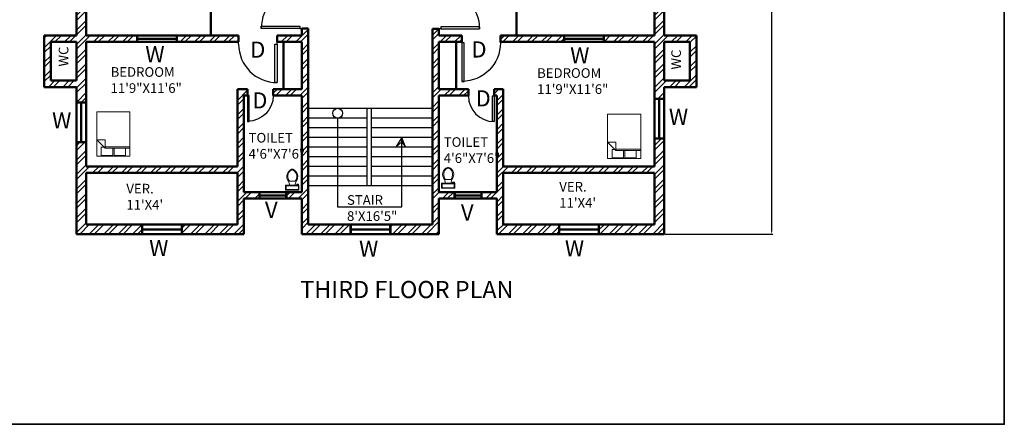
# Model space of a CAD drawing. Units: inches. Extents: x -31485 to -28799, y 18003 to 19130.
# Tile 11 of 15: x -29717 to -28799, y 18003 to 18380. Entities that reach past the tile are written whole.
import ezdxf

# ---------------------------------------------------------------- set-up
doc = ezdxf.new("R2010")
doc.units = ezdxf.units.IN
for name, color, linetype, lineweight in [('A-ANNO-DIMS', 2, 'Continuous', 18), ('A-ANNO-TEXT', 7, 'Continuous', 18), ('A-ANNO-TTLB', 7, 'Continuous', 35), ('A-AREA-IDEN', 7, 'Continuous', 18), ('A-DOOR', 3, 'Continuous', 25), ('A-FLOR-FIXT', 9, 'Continuous', 18), ('A-FLOR-STRS', 3, 'Continuous', 25), ('A-FURN', 8, 'Continuous', 18), ('A-GLAZ', 4, 'Continuous', 25), ('A-WALL', 7, 'Continuous', 50), ('A-WALL-PATT', 8, 'Continuous', 13)]:
    doc.layers.add(name, color=color, linetype=linetype, lineweight=lineweight)
doc.styles.get("Standard").update_dxf_attribs({"font": 'arial.ttf'})
doc.dimstyles.new('ISO-25', dxfattribs={"dimtxt": 2.5, "dimasz": 2.5, "dimexe": 1.25, "dimexo": 0.625, "dimtad": 1, "dimdec": 0, "dimlunit": 3, "dimtxsty": 'Standard', "dimcen": 2.5, "dimadec": 0, "dimazin": 0, "dimtfac": 1, "dimtdec": 0, "dimtmove": 0, "dimatfit": 3, "dimfxl": 1, "dimarcsym": 0})

# ---------------------------------------------------------------- blocks, each defined once
blk = doc.blocks.new('*U8')
for p, q in [((0, 0), (0, -100)), ((750, 0), (750, -100))]:
    blk.add_line(p, q)
blk.add_lwpolyline([(0, 0), (0, 750), (43.75, 750), (43.75, 0)], close=True)
blk.add_arc((0, 0), 750, 0, 90)
blk = doc.blocks.new('Bed - Queen')
for p, q in [((0, -80.00003), (0, 0)), ((0, 0), (59.99999, 0)), ((59.99999, 0), (59.99999, -80.00003)), ((0, -14.4), (44.8, -14.4)), ((44.8, -16.8), (0, -16.8)), ((7.99999, -1.2), (28.79998, -1.2)), ((7.99999, -14.4), (7.99999, -1.2)), ((28.79998, -1.2), (28.79998, -14.4)), ((31.19999, -1.2), (51.99999, -1.2)), ((31.19999, -14.4), (31.19999, -1.2)), ((59.99999, -29.6), (44.8, -14.4)), ((44.8, -14.4), (44.8, -29.6)), ((51.99999, -16.4), (46.79936, -16.4)), ((51.99999, -1.2), (51.99999, -16.4)), ((44.8, -29.6), (59.99999, -29.6)), ((59.99999, -80.00003), (0, -80.00003))]:
    blk.add_line(p, q)
blk = doc.blocks.new('Toilet - top')
for p, q in [((-10, -8.5), (-8, -8.5)), ((-10, -9.5), (-10, -8.5)), ((-7, -9.5), (-10, -9.5)), ((-8, -8.5), (-8, -8)), ((-7, -8), (-7, -9.5)), ((-4, -8), (-6, -14)), ((4, -14), (-4, -14)), ((4, -8), (6, -14)), ((9.5, -6), (9.5, -2))]:
    blk.add_line(p, q)
blk.add_lwpolyline([(10.5, -8), (10.5, 0), (-10.5, 0), (-10.5, -8)], close=True)
for points in [[(-9.5, -2), (-9.5, -6)], [(8.5, -1), (-8.5, -1)], [(-8.5, -7), (8.5, -7)]]:
    blk.add_lwpolyline(points)
for centre, radius, start, end in [((-8.6, -1.9), 0.884, 81.8699, 188.1301), ((-8.6, -6.1), 0.884, 171.8699, 278.1301), ((3.5, -21.6), 12.2, 141.4691, 247.9714), ((4.2, -21.8), 11.3, 136.3677, 238.9468), ((-3.5, -21.6), 12.2, 292.0284, 38.5307), ((-4.2, -21.8), 11.3, 301.053, 43.6321), ((8.6, -1.9), 0.884, 351.8699, 98.1301), ((8.6, -6.1), 0.884, 261.8699, 8.1301), ((0, -27.9), 4, 245.7318, 294.2682), ((0, -29), 4, 254.8605, 285.1395)]:
    blk.add_arc(centre, radius, start, end)
blk = doc.blocks.new('*D205')
at = {"layer": 'A-ANNO-DIMS', "color": 0, "lineweight": -2, "transparency": 16777216}
for p, q in [((-29115.2, 18824.12), (-29014.56, 18824.12)), ((-29015.81, 18821.62), (-29015.81, 18182.62)), ((-29115.2, 18180.12), (-29014.56, 18180.12))]:
    blk.add_line(p, q, dxfattribs=at)
at = {"layer": 'A-ANNO-DIMS', "color": 0, "transparency": 16777216}
for points in [[(-29016.23, 18821.62), (-29015.4, 18821.62), (-29015.81, 18824.12)], [(-29016.23, 18182.62), (-29015.4, 18182.62), (-29015.81, 18180.12)]]:
    blk.add_solid(points, dxfattribs=at)
at = {"layer": 'Defpoints', "color": 0, "transparency": 16777216}
for p in [(-29115.82, 18824.12), (-29115.82, 18180.12), (-29015.81, 18180.12)]:
    blk.add_point(p, dxfattribs=at)
at = {"layer": 'A-ANNO-DIMS', "color": 0, "transparency": 16777216, "insert": (-29024.61, 18502.12), "char_height": 2.5, "attachment_point": 5, "rotation": 90}
blk.add_mtext('{\\H6.4x;53\'-8"}', dxfattribs=at)
blk = doc.blocks.new('WIN-900-W9')
for p, q in [((-29982.21, 18824.12), (-29982.21, 18815.12)), ((-29981.21, 18824.12), (-29981.21, 18815.12)), ((-29945.21, 18824.12), (-29945.21, 18815.12)), ((-29944.21, 18824.12), (-29944.21, 18815.12)), ((-29981.21, 18820.12), (-29945.21, 18820.12)), ((-29981.21, 18819.62), (-29945.21, 18819.62)), ((-29981.21, 18819.12), (-29945.21, 18819.12))]:
    blk.add_line(p, q)
blk = doc.blocks.new('WIN-900-W6')
for p, q in [((-30183.21, 18720.12), (-30177.21, 18720.12)), ((-30183.21, 18719.12), (-30177.21, 18719.12)), ((-30180.71, 18683.12), (-30180.71, 18719.12)), ((-30180.21, 18683.12), (-30180.21, 18719.12)), ((-30179.71, 18683.12), (-30179.71, 18719.12)), ((-30183.21, 18683.12), (-30177.21, 18683.12)), ((-30183.21, 18682.12), (-30177.21, 18682.12))]:
    blk.add_line(p, q)
blk = doc.blocks.new('VENT-600-W6')
for p, q in [((-29884.21, 18519.12), (-29878.21, 18519.12)), ((-29884.21, 18518.12), (-29878.21, 18518.12)), ((-29881.71, 18494.12), (-29881.71, 18518.12)), ((-29881.21, 18494.12), (-29881.21, 18518.12)), ((-29880.71, 18494.12), (-29880.71, 18518.12)), ((-29884.21, 18494.12), (-29878.21, 18494.12)), ((-29884.21, 18493.12), (-29878.21, 18493.12))]:
    blk.add_line(p, q)

msp = doc.modelspace()

# ---------------------------------------------------------------- hatches: boundary and pattern name
at = {"layer": 'A-WALL-PATT'}
h = msp.add_hatch(dxfattribs=at)
h.set_pattern_fill('ANSI32', color=256)
h.set_pattern_definition([(45, (-227.67, 0), (-6.735192, 6.735192), []), (45, (-223.18, 0), (-6.735192, 6.735192), [])])
h.paths.add_polyline_path([(-29507.82, 18213.12), (-29493.82, 18213.12), (-29493.82, 18219.12), (-29507.82, 18219.12), (-29507.82, 18309.12), (-29504.3, 18309.12), (-29504.3, 18315.12), (-29513.82, 18315.12), (-29513.82, 18243.12), (-29654.82, 18243.12), (-29654.82, 18265.36), (-29663.82, 18265.36), (-29663.82, 18180.12), (-29603.32, 18180.12), (-29603.32, 18189.12), (-29654.82, 18189.12), (-29654.82, 18237.12), (-29513.82, 18237.12), (-29513.82, 18189.12), (-29565.32, 18189.12), (-29565.32, 18180.12), (-29507.82, 18180.12)])
h.paths.add_polyline_path([(-29408.82, 18189.12), (-29447.82, 18189.12), (-29447.82, 18371.74), (-29453.82, 18371.74), (-29453.82, 18365.12), (-29476.66, 18365.12), (-29476.66, 18359.12), (-29453.82, 18359.12), (-29453.82, 18315.12), (-29480.3, 18315.12), (-29480.3, 18309.12), (-29453.82, 18309.12), (-29453.82, 18219.12), (-29467.82, 18219.12), (-29467.82, 18213.12), (-29453.82, 18213.12), (-29453.82, 18180.12), (-29408.82, 18180.12)])
h.paths.add_polyline_path([(-29325.82, 18213.12), (-29311.82, 18213.12), (-29311.82, 18219.12), (-29325.82, 18219.12), (-29325.82, 18309.12), (-29298.35, 18309.12), (-29298.35, 18315.12), (-29325.82, 18315.12), (-29325.82, 18359.12), (-29304.41, 18359.12), (-29304.41, 18365.12), (-29325.82, 18365.12), (-29325.82, 18371.25), (-29331.82, 18371.25), (-29331.82, 18189.12), (-29370.82, 18189.12), (-29370.82, 18180.12), (-29325.82, 18180.12)])
h.paths.add_polyline_path([(-29265.82, 18237.12), (-29124.82, 18237.12), (-29124.82, 18189.12), (-29176.32, 18189.12), (-29176.32, 18180.12), (-29115.82, 18180.12), (-29115.82, 18268.84), (-29124.82, 18268.84), (-29124.82, 18243.12), (-29265.82, 18243.12), (-29265.82, 18315.12), (-29274.35, 18315.12), (-29274.35, 18309.12), (-29271.82, 18309.12), (-29271.82, 18219.12), (-29285.82, 18219.12), (-29285.82, 18213.12), (-29271.82, 18213.12), (-29271.82, 18180.12), (-29214.32, 18180.12), (-29214.32, 18189.12), (-29265.82, 18189.12)])
h.paths.add_polyline_path([(-29209.82, 18365.12), (-29262.82, 18365.12), (-29268.41, 18365.12), (-29268.41, 18359.12), (-29209.82, 18359.12)])
h.paths.add_polyline_path([(-29085.82, 18365.12), (-29115.82, 18365.12), (-29115.82, 18400.12), (-29124.82, 18400.12), (-29124.82, 18365.12), (-29171.82, 18365.12), (-29171.82, 18359.12), (-29124.82, 18359.12), (-29124.82, 18306.84), (-29115.82, 18306.84), (-29115.82, 18317.12), (-29085.82, 18317.12)])
h.paths.add_polyline_path([(-29115.82, 18359.12), (-29091.82, 18359.12), (-29091.82, 18323.12), (-29115.82, 18323.12)], flags=16)
h.paths.add_polyline_path([(-29607.82, 18365.12), (-29654.82, 18365.12), (-29654.82, 18400.12), (-29663.82, 18400.12), (-29663.82, 18365.12), (-29693.82, 18365.12), (-29693.82, 18317.12), (-29663.82, 18317.12), (-29663.82, 18303.36), (-29654.82, 18303.36), (-29654.82, 18359.12), (-29607.82, 18359.12)])
h.paths.add_polyline_path([(-29663.82, 18359.12), (-29663.82, 18323.12), (-29687.82, 18323.12), (-29687.82, 18359.12)], flags=16)
h.paths.add_polyline_path([(-29512.66, 18365.12), (-29516.82, 18365.12), (-29569.82, 18365.12), (-29569.82, 18359.12), (-29512.66, 18359.12)])
h.paths.add_polyline_path([(-29654.82, 18473.12), (-29553.73, 18473.12), (-29553.73, 18479.12), (-29564.82, 18479.12), (-29564.82, 18500.25), (-29569.57, 18500.25, -0.011537), (-29570.67, 18500.25), (-29570.82, 18500.25), (-29570.82, 18479.12), (-29675.82, 18479.12), (-29675.82, 18493.12), (-29681.82, 18493.12), (-29681.82, 18473.12), (-29663.82, 18473.12), (-29663.82, 18438.12), (-29654.82, 18438.12)])
h.paths.add_polyline_path([(-29564.82, 18547.44), (-29570.82, 18547.44), (-29570.82, 18539.12), (-29654.82, 18539.12), (-29654.82, 18562.12), (-29663.82, 18562.12), (-29663.82, 18539.12), (-29681.82, 18539.12), (-29681.82, 18519.12), (-29675.82, 18519.12), (-29675.82, 18533.12), (-29570.82, 18533.12), (-29570.82, 18524.25), (-29564.82, 18524.25)])
h.paths.add_polyline_path([(-29563.19, 18629.12), (-29654.82, 18629.12), (-29654.82, 18682.12), (-29663.82, 18682.12), (-29663.82, 18600.12), (-29654.82, 18600.12), (-29654.82, 18623.12), (-29570.82, 18623.12), (-29570.82, 18583.44), (-29566.85, 18583.44), (-29564.82, 18583.44), (-29564.82, 18623.12), (-29563.19, 18623.12)])
h.paths.add_polyline_path([(-29315.33, 18629.12), (-29396.82, 18629.12), (-29396.82, 18682.12), (-29402.82, 18682.12), (-29402.82, 18629.12), (-29482.28, 18629.12), (-29482.28, 18626.12), (-29482.28, 18623.12), (-29402.82, 18623.12), (-29402.82, 18416.12), (-29453.82, 18416.12), (-29453.82, 18407.74), (-29447.82, 18407.74), (-29447.82, 18410.12), (-29331.82, 18410.12), (-29331.82, 18407.25), (-29325.82, 18407.25), (-29325.82, 18416.12), (-29396.82, 18416.12), (-29396.82, 18623.12), (-29315.33, 18623.12)])
h.paths.add_polyline_path([(-29525.82, 18773.12), (-29492.32, 18773.12), (-29492.32, 18779.12), (-29498.82, 18779.12), (-29498.82, 18815.12), (-29469.82, 18815.12), (-29469.82, 18824.12), (-29504.82, 18824.12), (-29504.82, 18779.12), (-29552.82, 18779.12), (-29552.82, 18824.12), (-29587.82, 18824.12), (-29587.82, 18815.12), (-29558.82, 18815.12), (-29558.82, 18779.12), (-29563.08, 18779.12), (-29563.08, 18776.12), (-29563.08, 18773.12), (-29531.82, 18773.12), (-29531.82, 18629.12), (-29533.3, 18629.12), (-29533.3, 18626.12), (-29533.3, 18623.12), (-29518.28, 18623.12), (-29518.28, 18629.12), (-29525.82, 18629.12)])
h.paths.add_polyline_path([(-29654.82, 18779.12), (-29654.82, 18815.12), (-29625.82, 18815.12), (-29625.82, 18824.12), (-29663.82, 18824.12), (-29663.82, 18779.12), (-29693.82, 18779.12), (-29693.82, 18731.12), (-29663.82, 18731.12), (-29663.82, 18720.12), (-29654.82, 18720.12), (-29654.82, 18773.12), (-29587.08, 18773.12), (-29587.08, 18779.12)])
h.paths.add_polyline_path([(-29663.82, 18773.12), (-29663.82, 18737.12), (-29687.82, 18737.12), (-29687.82, 18773.12)], flags=16)
h.paths.add_polyline_path([(-29396.82, 18815.12), (-29367.82, 18815.12), (-29367.82, 18824.12), (-29431.82, 18824.12), (-29431.82, 18815.12), (-29402.82, 18815.12), (-29402.82, 18779.12), (-29468.32, 18779.12), (-29468.32, 18776.12), (-29468.32, 18773.12), (-29402.82, 18773.12), (-29402.82, 18720.12), (-29396.82, 18720.12), (-29396.82, 18773.12), (-29331.17, 18773.12), (-29331.17, 18779.12), (-29396.82, 18779.12)])
h.paths.add_polyline_path([(-29232.68, 18779.12), (-29240.82, 18779.12), (-29240.82, 18815.12), (-29201.82, 18815.12), (-29201.82, 18824.12), (-29246.82, 18824.12), (-29246.82, 18779.12), (-29294.82, 18779.12), (-29294.82, 18824.12), (-29329.82, 18824.12), (-29329.82, 18815.12), (-29300.82, 18815.12), (-29300.82, 18779.12), (-29307.17, 18779.12), (-29307.17, 18776.12), (-29307.17, 18773.12), (-29273.82, 18773.12), (-29273.82, 18629.12), (-29279.33, 18629.12), (-29279.33, 18626.12), (-29279.33, 18623.12), (-29262.04, 18623.12), (-29262.04, 18629.12), (-29267.82, 18629.12), (-29267.82, 18773.12), (-29232.68, 18773.12)])
h.paths.add_polyline_path([(-29085.82, 18779.12), (-29115.82, 18779.12), (-29115.82, 18824.12), (-29163.82, 18824.12), (-29163.82, 18815.12), (-29124.82, 18815.12), (-29124.82, 18779.12), (-29208.68, 18779.12), (-29208.68, 18776.12), (-29208.68, 18773.12), (-29124.82, 18773.12), (-29124.82, 18720.12), (-29115.82, 18720.12), (-29115.82, 18731.12), (-29085.82, 18731.12)])
h.paths.add_polyline_path([(-29115.82, 18773.12), (-29091.82, 18773.12), (-29091.82, 18737.12), (-29115.82, 18737.12)], flags=16)
h.paths.add_polyline_path([(-29115.82, 18682.12), (-29124.82, 18682.12), (-29124.82, 18629.12), (-29226.04, 18629.12), (-29226.04, 18626.12), (-29226.04, 18623.12), (-29214.82, 18623.12), (-29214.82, 18589.35), (-29208.82, 18589.35), (-29208.82, 18623.12), (-29124.82, 18623.12), (-29124.82, 18600.12), (-29115.82, 18600.12)])
h.paths.add_polyline_path([(-29115.82, 18562.12), (-29124.82, 18562.12), (-29124.82, 18539.12), (-29208.82, 18539.12), (-29208.82, 18553.35), (-29211.82, 18553.35), (-29214.82, 18553.35), (-29214.82, 18522.99), (-29208.82, 18522.99), (-29208.82, 18533.12), (-29103.82, 18533.12), (-29103.82, 18519.12), (-29097.82, 18519.12), (-29097.82, 18539.12), (-29115.82, 18539.12)])
h.paths.add_polyline_path([(-29115.82, 18473.12), (-29097.82, 18473.12), (-29097.82, 18493.12), (-29103.82, 18493.12), (-29103.82, 18479.12), (-29208.82, 18479.12), (-29208.82, 18498.99), (-29214.82, 18498.99), (-29214.82, 18479.12), (-29238.82, 18479.12), (-29238.82, 18473.12), (-29124.82, 18473.12), (-29124.82, 18438.12), (-29115.82, 18438.12)])
h.paths.add_polyline_path([(-29513.85, 18245.24), (-29448.79, 18245.24), (-29448.79, 18278.82), (-29513.85, 18278.82)], flags=9)
h.paths.add_polyline_path([(-29331.85, 18241.25), (-29266.79, 18241.25), (-29266.79, 18274.84), (-29331.85, 18274.84)], flags=9)
h.paths.add_polyline_path([(-29095.1, 18330.99), (-29095.1, 18356.44), (-29113.65, 18356.44), (-29113.65, 18330.99)], flags=8)
h.paths.add_polyline_path([(-29666.32, 18333.81), (-29666.32, 18359.25), (-29684.87, 18359.25), (-29684.87, 18333.81)], flags=24)
h.paths.add_polyline_path([(-29665.76, 18745.92), (-29665.76, 18771.37), (-29684.31, 18771.37), (-29684.31, 18745.92)], flags=8)
h.paths.add_polyline_path([(-29093.62, 18744.62), (-29093.62, 18770.06), (-29112.17, 18770.06), (-29112.17, 18744.62)], flags=8)

# ---------------------------------------------------------------- linework, layer by layer
at = {"layer": 'A-ANNO-TTLB'}
msp.add_lwpolyline([(-31485.1, 19129.94), (-28798.64, 19129.94), (-28798.64, 18002.86), (-31485.1, 18002.86)], close=True, dxfattribs=at)
at = {"layer": 'A-FLOR-STRS'}
for p, q in [((-29331.82, 18297.12), (-29447.82, 18297.12)), ((-29392.82, 18225.12), (-29392.82, 18297.12)), ((-29388.82, 18225.12), (-29388.82, 18297.12)), ((-29392.82, 18288.12), (-29447.82, 18288.12)), ((-29420.32, 18288.12), (-29420.32, 18205.58)), ((-29331.82, 18288.12), (-29388.82, 18288.12)), ((-29392.82, 18279.12), (-29447.82, 18279.12)), ((-29331.82, 18279.12), (-29388.82, 18279.12)), ((-29392.82, 18270.12), (-29447.82, 18270.12)), ((-29331.82, 18270.12), (-29388.82, 18270.12)), ((-29360.32, 18270.12), (-29365.89, 18261.12)), ((-29365.89, 18261.12), (-29360.32, 18265.99)), ((-29360.32, 18205.58), (-29360.32, 18270.12)), ((-29357.14, 18261.12), (-29360.32, 18270.12)), ((-29360.32, 18265.99), (-29357.14, 18261.12)), ((-29392.82, 18261.12), (-29447.82, 18261.12)), ((-29331.82, 18261.12), (-29388.82, 18261.12)), ((-29392.82, 18252.12), (-29447.82, 18252.12)), ((-29331.82, 18252.12), (-29388.82, 18252.12)), ((-29392.82, 18243.12), (-29447.82, 18243.12)), ((-29331.82, 18243.12), (-29388.82, 18243.12)), ((-29392.82, 18234.12), (-29447.82, 18234.12)), ((-29331.82, 18234.12), (-29388.82, 18234.12)), ((-29331.82, 18225.12), (-29447.82, 18225.12)), ((-29420.32, 18205.58), (-29360.32, 18205.58))]:
    msp.add_line(p, q, dxfattribs=at)
msp.add_circle((-29420.32, 18292.7), 4.58, dxfattribs=at)
at = {"layer": 'A-WALL'}
for p, q in [((-29538.64, 18476.12), (-29538.64, 18365.12)), ((-29253.51, 18476.12), (-29253.51, 18365.12)), ((-29663.82, 18365.12), (-29663.82, 18473.12)), ((-29654.82, 18365.12), (-29654.82, 18473.12)), ((-29124.82, 18473.12), (-29124.82, 18365.12)), ((-29115.82, 18473.12), (-29115.82, 18365.12)), ((-29693.82, 18365.12), (-29663.82, 18365.12)), ((-29693.82, 18317.12), (-29693.82, 18365.12)), ((-29654.82, 18365.12), (-29516.82, 18365.12)), ((-29516.82, 18365.12), (-29512.66, 18365.12)), ((-29512.66, 18365.12), (-29512.66, 18359.12)), ((-29476.66, 18365.12), (-29476.66, 18359.12)), ((-29476.66, 18365.12), (-29453.82, 18365.12)), ((-29453.82, 18365.12), (-29453.82, 18371.74)), ((-29453.82, 18371.74), (-29447.82, 18371.74)), ((-29447.82, 18189.12), (-29447.82, 18371.74)), ((-29331.82, 18371.25), (-29325.82, 18371.25)), ((-29331.82, 18371.25), (-29331.82, 18189.12)), ((-29325.82, 18371.25), (-29325.82, 18365.12)), ((-29325.82, 18365.12), (-29304.41, 18365.12)), ((-29304.41, 18365.12), (-29304.41, 18359.12)), ((-29268.41, 18365.12), (-29268.41, 18359.12)), ((-29268.41, 18365.12), (-29262.82, 18365.12)), ((-29262.82, 18365.12), (-29124.82, 18365.12)), ((-29115.82, 18365.12), (-29085.82, 18365.12)), ((-29085.82, 18365.12), (-29085.82, 18317.12)), ((-29687.82, 18359.12), (-29663.82, 18359.12)), ((-29687.82, 18323.12), (-29687.82, 18359.12)), ((-29663.82, 18323.12), (-29663.82, 18359.12)), ((-29654.82, 18243.12), (-29654.82, 18359.12)), ((-29654.82, 18359.12), (-29512.66, 18359.12)), ((-29476.66, 18359.12), (-29453.82, 18359.12)), ((-29470.66, 18359.12), (-29470.66, 18315.12)), ((-29453.82, 18315.12), (-29453.82, 18359.12)), ((-29325.82, 18359.12), (-29304.41, 18359.12)), ((-29325.82, 18359.12), (-29325.82, 18315.12)), ((-29309.71, 18359.12), (-29309.71, 18315.12)), ((-29268.41, 18359.12), (-29124.82, 18359.12)), ((-29124.82, 18359.12), (-29124.82, 18243.12)), ((-29115.82, 18359.12), (-29115.82, 18323.12)), ((-29115.82, 18359.12), (-29091.82, 18359.12)), ((-29091.82, 18359.12), (-29091.82, 18323.12)), ((-29687.82, 18323.12), (-29663.82, 18323.12)), ((-29115.82, 18323.12), (-29091.82, 18323.12)), ((-29693.82, 18317.12), (-29663.82, 18317.12)), ((-29663.82, 18180.12), (-29663.82, 18317.12)), ((-29513.82, 18243.12), (-29513.82, 18315.12)), ((-29504.3, 18315.12), (-29513.82, 18315.12)), ((-29507.82, 18219.12), (-29507.82, 18309.12)), ((-29504.3, 18309.12), (-29507.82, 18309.12)), ((-29504.3, 18315.12), (-29504.3, 18309.12)), ((-29453.82, 18315.12), (-29480.3, 18315.12)), ((-29480.3, 18315.12), (-29480.3, 18309.12)), ((-29453.82, 18309.12), (-29480.3, 18309.12)), ((-29453.82, 18219.12), (-29453.82, 18309.12)), ((-29298.35, 18315.12), (-29325.82, 18315.12)), ((-29325.82, 18309.12), (-29325.82, 18219.12)), ((-29298.35, 18309.12), (-29325.82, 18309.12)), ((-29298.35, 18315.12), (-29298.35, 18309.12)), ((-29265.82, 18315.12), (-29274.35, 18315.12)), ((-29274.35, 18315.12), (-29274.35, 18309.12)), ((-29271.82, 18309.12), (-29274.35, 18309.12)), ((-29271.82, 18309.12), (-29271.82, 18219.12)), ((-29265.82, 18315.12), (-29265.82, 18243.12)), ((-29115.82, 18317.12), (-29085.82, 18317.12)), ((-29115.82, 18317.12), (-29115.82, 18180.12)), ((-29513.82, 18243.12), (-29654.82, 18243.12)), ((-29654.82, 18189.12), (-29654.82, 18237.12)), ((-29513.82, 18237.12), (-29654.82, 18237.12)), ((-29513.82, 18189.12), (-29513.82, 18237.12)), ((-29124.82, 18243.12), (-29265.82, 18243.12)), ((-29124.82, 18237.12), (-29265.82, 18237.12)), ((-29265.82, 18237.12), (-29265.82, 18189.12)), ((-29124.82, 18237.12), (-29124.82, 18189.12)), ((-29453.82, 18219.12), (-29507.82, 18219.12)), ((-29271.82, 18219.12), (-29325.82, 18219.12)), ((-29507.82, 18180.12), (-29507.82, 18213.12)), ((-29453.82, 18213.12), (-29507.82, 18213.12)), ((-29453.82, 18180.12), (-29453.82, 18213.12)), ((-29271.82, 18213.12), (-29325.82, 18213.12)), ((-29325.82, 18213.12), (-29325.82, 18180.12)), ((-29271.82, 18213.12), (-29271.82, 18180.12)), ((-29513.82, 18189.12), (-29654.82, 18189.12)), ((-29331.82, 18189.12), (-29447.82, 18189.12)), ((-29124.82, 18189.12), (-29265.82, 18189.12)), ((-29507.82, 18180.12), (-29663.82, 18180.12)), ((-29325.82, 18180.12), (-29453.82, 18180.12)), ((-29115.82, 18180.12), (-29271.82, 18180.12))]:
    msp.add_line(p, q, dxfattribs=at)

# ---------------------------------------------------------------- block references
at = {"layer": 'A-DOOR'}
for p, xscale, yscale, zscale, rotation in [((-29455.56, 18371.7), 0.0480000000000013, 0.0480000000000013, 0.0480000000000013, 90.00000000000003), ((-29324.02, 18371.25), -0.0480000007307817, 0.0480000007307817, 0.0480000007307817, 270), ((-29476.71, 18357.13), 0.0478890251559745, 0.0478890251559745, 0.0478890251559745, 180), ((-29304.36, 18358.26), -0.047820759004354, 0.047820759004354, 0.047820759004354, 180), ((-29504.28, 18309.12), -0.0319658169262993, 0.0319658169262993, 0.0319658169262993, 180), ((-29274.35, 18308.88), 0.0319999824341765, 0.0319999824341765, 0.0319999824341765, 180)]:
    msp.add_blockref('*U8', p, dxfattribs=dict(at, xscale=xscale, yscale=yscale, zscale=zscale, rotation=rotation))
at = {"layer": 'A-FLOR-FIXT', "xscale": 0.5926017901613329, "yscale": 0.5926017901613329, "zscale": 0.5926017901613329, "rotation": 180}
for p in [(-29462.59, 18220.97), (-29317.24, 18222.73)]:
    msp.add_blockref('Toilet - top', p, dxfattribs=at)
at = {"layer": 'A-FURN', "xscale": 0.5144931166195136, "yscale": 0.5144931166195136, "zscale": 0.5144931166195136, "rotation": 180}
for p in [(-29613.98, 18252.75), (-29137.7, 18250.61)]:
    msp.add_blockref('Bed - Queen', p, dxfattribs=at)
at = {"layer": 'A-GLAZ'}
for name, p, rotation in [('WIN-900-W6', (-48289.94, -11818.09), 269.9999999999927), ('WIN-900-W6', (-47891.94, -11818.09), 270.000000000009), ('WIN-900-W9', (-10839.7, 48247.57), 89.9999999999743), ('WIN-900-W9', (-10300.7, 48251.05), 89.9999999999896), ('VENT-600-W6', (-47986.94, -11665.09), 269.9999999999977), ('VENT-600-W6', (-47804.94, -11665.09), 270.0000000000153)]:
    msp.add_blockref(name, p, dxfattribs=dict(at, rotation=rotation))
for p in [(378.88, -635), (573.38, -635), (767.88, -635)]:
    msp.add_blockref('WIN-900-W9', p, dxfattribs=at)

# ---------------------------------------------------------------- texts
at = {"layer": 'A-ANNO-TEXT', "attachment_point": 1}
for s, width, insert, char_height in [('{W}', 1534.0875, (-29599.65, 18355.21), 15), ('{D}', 1534.0875, (-29501.79, 18359.49), 15), ('{D}', 1534.0875, (-29295.51, 18359.63), 15), ('{W}', 1534.0875, (-29203.47, 18354.26), 15), ('{D}', 1534.0875, (-29499.9, 18312.12), 15), ('{D}', 1534.0875, (-29291.63, 18314.03), 15), ('{W}', 1534.0875, (-29686.58, 18293.53), 15), ('{W}', 1534.0875, (-29111.42, 18296.88), 15), ('{V}', 1534.0875, (-29488.03, 18210.17), 15), ('{V}', 1534.0875, (-29305.33, 18207.69), 15), ('{W}', 1534.0875, (-29596.07, 18174.7), 15), ('{W}', 1534.0875, (-29400.36, 18174.05), 15), ('{W}', 1534.0875, (-29208.42, 18174.41), 15), ('{THIRD FLOOR PLAN}', 2526.6929, (-29455.2, 18136.42), 16)]:
    msp.add_mtext_dynamic_manual_height_columns(s, width=width, gutter_width=12.5, heights=[0], dxfattribs=dict(at, insert=insert, char_height=char_height))
at = {"layer": 'A-AREA-IDEN', "char_height": 9, "attachment_point": 1, "rotation": 90}
for insert in [(-29680.39, 18336.21), (-29109.17, 18333.39)]:
    msp.add_mtext_dynamic_manual_height_columns('{WC}', width=988.498, gutter_width=12.5, heights=[0], dxfattribs=dict(at, insert=insert))
at = {"layer": 'A-AREA-IDEN', "char_height": 9, "attachment_point": 1}
for s, insert in [('{BEDROOM\\P11\'9"X11\'6"}', (-29631.99, 18335.63)), ('{ BEDROOM\\P 11\'9"X11\'6"}', (-29237.02, 18334.68)), ('{   TOILET\\P   4\'6"X7\'6"}', (-29511.6, 18274.35)), ('{   TOILET\\P   4\'6"X7\'6"}', (-29329.6, 18270.37)), ("{VER.\\P11'X4'}", (-29617.32, 18226.92)), ("{     VER.\\P     11'X4'}", (-29227.38, 18228.73)), ('{  STAIR\\P  8\'X16\'5"}', (-29417.07, 18216.37))]:
    msp.add_mtext_dynamic_manual_height_columns(s, width=988.498, gutter_width=12.5, heights=[0], dxfattribs=dict(at, insert=insert))

# ---------------------------------------------------------------- dimensions: what is measured, and where the dimension line sits
at = {"layer": 'A-ANNO-DIMS'}
dim = msp.add_linear_dim(base=(-29015.81, 18180.12), p1=(-29115.82, 18824.12), p2=(-29115.82, 18180.12), angle=90, text='{\\H6.4x;<>}', dimstyle='ISO-25', override={"dimclrd": 0, "dimclre": 0, "dimclrt": 0}, dxfattribs=at)
dim.commit()
dim.dimension.update_dxf_attribs({"geometry": '*D205', "text_midpoint": (-29024.61, 18502.12)})

doc.saveas('drawing.dxf')
